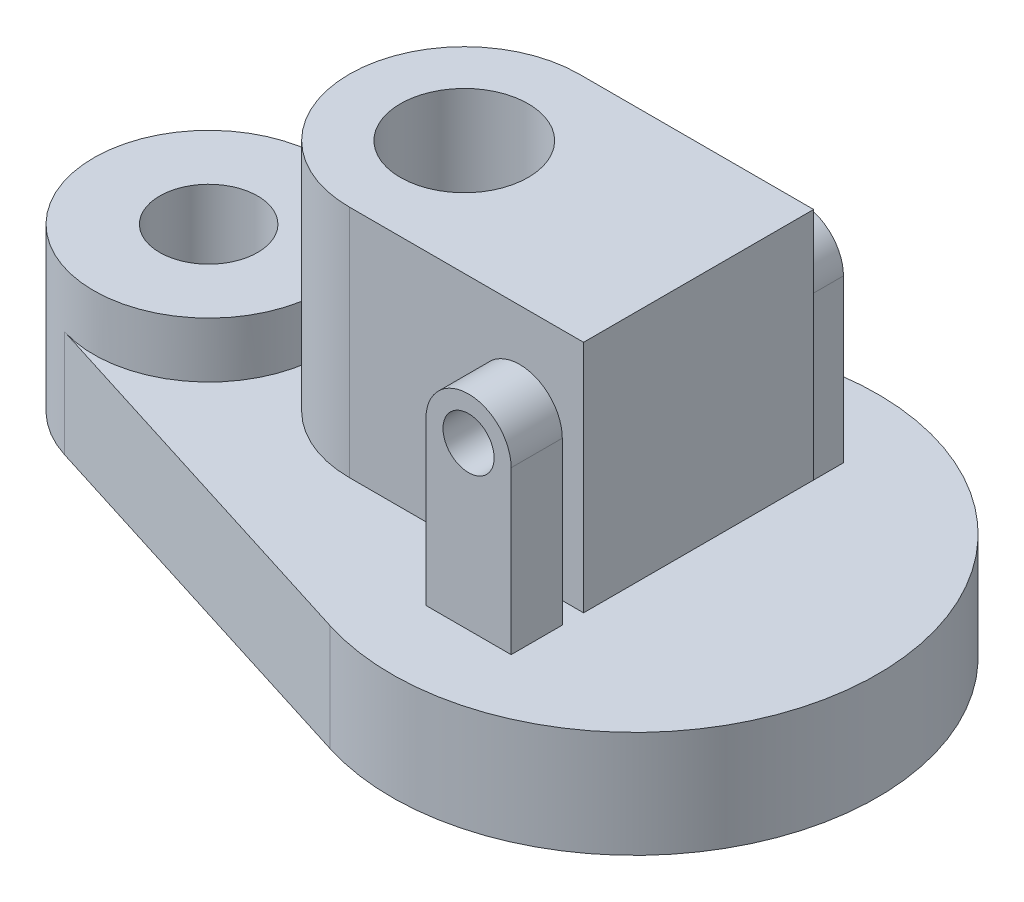
ISO-10303-21;
HEADER;
FILE_DESCRIPTION(('STEP AP214'),'2;1');
FILE_NAME('part.step','',(''),(''),'','','');
FILE_SCHEMA(('AUTOMOTIVE_DESIGN { 1 0 10303 214 1 1 1 1 }'));
ENDSEC;
DATA;
#1=APPLICATION_CONTEXT('core data for automotive mechanical design processes');
#2=APPLICATION_PROTOCOL_DEFINITION('international standard','automotive_design',2000,#1);
#3=PRODUCT_CONTEXT('',#1,'mechanical');
#4=PRODUCT('Part','Part','',(#3));
#5=PRODUCT_RELATED_PRODUCT_CATEGORY('part','',(#4));
#6=PRODUCT_DEFINITION_FORMATION('','',#4);
#7=PRODUCT_DEFINITION_CONTEXT('part definition',#1,'design');
#8=PRODUCT_DEFINITION('design','',#6,#7);
#9=PRODUCT_DEFINITION_SHAPE('','',#8);
#10=(LENGTH_UNIT() NAMED_UNIT(*) SI_UNIT(.MILLI.,.METRE.));
#11=(NAMED_UNIT(*) PLANE_ANGLE_UNIT() SI_UNIT($,.RADIAN.));
#12=(NAMED_UNIT(*) SI_UNIT($,.STERADIAN.) SOLID_ANGLE_UNIT());
#13=UNCERTAINTY_MEASURE_WITH_UNIT(LENGTH_MEASURE(1.E-05),#10,'distance_accuracy_value','');
#14=(GEOMETRIC_REPRESENTATION_CONTEXT(3) GLOBAL_UNCERTAINTY_ASSIGNED_CONTEXT((#13)) GLOBAL_UNIT_ASSIGNED_CONTEXT((#10,
#11,#12)) REPRESENTATION_CONTEXT('',''));
#15=CARTESIAN_POINT('',(0.,0.,0.));
#16=DIRECTION('',(0.,0.,1.));
#17=DIRECTION('',(1.,0.,0.));
#18=AXIS2_PLACEMENT_3D('',#15,#16,#17);
#19=CARTESIAN_POINT('',(0.,25.,0.));
#20=DIRECTION('',(0.,1.,0.));
#21=DIRECTION('',(0.,0.,1.));
#22=AXIS2_PLACEMENT_3D('',#19,#20,#21);
#23=PLANE('',#22);
#24=DIRECTION('',(0.953939201416946,0.,-0.3));
#25=VECTOR('',#24,1.);
#26=CARTESIAN_POINT('',(-17.1,25.,-54.3745344807659));
#27=LINE('',#26,#25);
#28=CARTESIAN_POINT('',(-108.1,25.,-25.7563584382575));
#29=VERTEX_POINT('',#28);
#30=CARTESIAN_POINT('',(-17.1,25.,-54.3745344807659));
#31=VERTEX_POINT('',#30);
#32=EDGE_CURVE('E247',#29,#31,#27,.T.);
#33=ORIENTED_EDGE('',*,*,#32,.F.);
#34=CARTESIAN_POINT('',(-100.,25.,0.));
#35=DIRECTION('',(0.,1.,0.));
#36=DIRECTION('',(0.,0.,1.));
#37=AXIS2_PLACEMENT_3D('',#34,#35,#36);
#38=CIRCLE('',#37,27.);
#39=CARTESIAN_POINT('',(-108.1,25.,25.7563584382575));
#40=VERTEX_POINT('',#39);
#41=EDGE_CURVE('E232',#29,#40,#38,.F.);
#42=ORIENTED_EDGE('',*,*,#41,.T.);
#43=DIRECTION('',(0.953939201416946,0.,0.3));
#44=VECTOR('',#43,1.);
#45=CARTESIAN_POINT('',(-17.1,25.,54.3745344807659));
#46=LINE('',#45,#44);
#47=CARTESIAN_POINT('',(-17.1,25.,54.3745344807659));
#48=VERTEX_POINT('',#47);
#49=EDGE_CURVE('E257',#40,#48,#46,.T.);
#50=ORIENTED_EDGE('',*,*,#49,.T.);
#51=CARTESIAN_POINT('',(0.,25.,0.));
#52=DIRECTION('',(0.,1.,0.));
#53=DIRECTION('',(0.,0.,1.));
#54=AXIS2_PLACEMENT_3D('',#51,#52,#53);
#55=CIRCLE('',#54,57.);
#56=EDGE_CURVE('E256',#48,#31,#55,.T.);
#57=ORIENTED_EDGE('',*,*,#56,.T.);
#58=EDGE_LOOP('',(#33,#42,#50,#57));
#59=FACE_BOUND('',#58,.T.);
#60=CARTESIAN_POINT('',(-40.,25.,0.));
#61=DIRECTION('',(0.,1.,0.));
#62=DIRECTION('',(0.,0.,1.));
#63=AXIS2_PLACEMENT_3D('',#60,#61,#62);
#64=CIRCLE('',#63,12.5);
#65=CARTESIAN_POINT('',(-40.,25.,12.5));
#66=VERTEX_POINT('',#65);
#67=EDGE_CURVE('E223',#66,#66,#64,.T.);
#68=ORIENTED_EDGE('',*,*,#67,.F.);
#69=EDGE_LOOP('',(#68));
#70=FACE_BOUND('',#69,.T.);
#71=DIRECTION('',(0.,0.,-1.));
#72=VECTOR('',#71,1.);
#73=CARTESIAN_POINT('',(10.,25.,39.));
#74=LINE('',#73,#72);
#75=CARTESIAN_POINT('',(10.,25.,39.));
#76=VERTEX_POINT('',#75);
#77=CARTESIAN_POINT('',(10.,25.,27.));
#78=VERTEX_POINT('',#77);
#79=EDGE_CURVE('E283',#76,#78,#74,.T.);
#80=ORIENTED_EDGE('',*,*,#79,.F.);
#81=DIRECTION('',(1.,0.,0.));
#82=VECTOR('',#81,1.);
#83=CARTESIAN_POINT('',(10.,25.,39.));
#84=LINE('',#83,#82);
#85=CARTESIAN_POINT('',(-10.,25.,39.));
#86=VERTEX_POINT('',#85);
#87=EDGE_CURVE('E282',#86,#76,#84,.T.);
#88=ORIENTED_EDGE('',*,*,#87,.F.);
#89=DIRECTION('',(0.,0.,-1.));
#90=VECTOR('',#89,1.);
#91=CARTESIAN_POINT('',(-10.,25.,39.));
#92=LINE('',#91,#90);
#93=CARTESIAN_POINT('',(-10.,25.,27.));
#94=VERTEX_POINT('',#93);
#95=EDGE_CURVE('E300',#86,#94,#92,.T.);
#96=ORIENTED_EDGE('',*,*,#95,.T.);
#97=DIRECTION('',(1.,0.,0.));
#98=VECTOR('',#97,1.);
#99=CARTESIAN_POINT('',(10.,25.,27.));
#100=LINE('',#99,#98);
#101=EDGE_CURVE('E280',#94,#78,#100,.T.);
#102=ORIENTED_EDGE('',*,*,#101,.T.);
#103=EDGE_LOOP('',(#80,#88,#96,#102));
#104=FACE_BOUND('',#103,.T.);
#105=DIRECTION('',(0.,0.,1.));
#106=VECTOR('',#105,1.);
#107=CARTESIAN_POINT('',(-9.99999999999999,25.,-39.));
#108=LINE('',#107,#106);
#109=CARTESIAN_POINT('',(-9.99999999999999,25.,-39.));
#110=VERTEX_POINT('',#109);
#111=CARTESIAN_POINT('',(-10.,25.,-27.));
#112=VERTEX_POINT('',#111);
#113=EDGE_CURVE('E218',#110,#112,#108,.T.);
#114=ORIENTED_EDGE('',*,*,#113,.F.);
#115=DIRECTION('',(1.,0.,0.));
#116=VECTOR('',#115,1.);
#117=CARTESIAN_POINT('',(-67.,25.,-39.));
#118=LINE('',#117,#116);
#119=CARTESIAN_POINT('',(9.99999999999999,25.,-39.));
#120=VERTEX_POINT('',#119);
#121=EDGE_CURVE('E187',#110,#120,#118,.T.);
#122=ORIENTED_EDGE('',*,*,#121,.T.);
#123=DIRECTION('',(0.,0.,1.));
#124=VECTOR('',#123,1.);
#125=CARTESIAN_POINT('',(9.99999999999999,25.,-39.));
#126=LINE('',#125,#124);
#127=CARTESIAN_POINT('',(9.99999999999999,25.,-27.));
#128=VERTEX_POINT('',#127);
#129=EDGE_CURVE('E199',#120,#128,#126,.T.);
#130=ORIENTED_EDGE('',*,*,#129,.T.);
#131=DIRECTION('',(1.,0.,0.));
#132=VECTOR('',#131,1.);
#133=CARTESIAN_POINT('',(-67.,25.,-27.));
#134=LINE('',#133,#132);
#135=EDGE_CURVE('E203',#112,#128,#134,.T.);
#136=ORIENTED_EDGE('',*,*,#135,.F.);
#137=EDGE_LOOP('',(#114,#122,#130,#136));
#138=FACE_BOUND('',#137,.T.);
#139=ADVANCED_FACE('F50',(#59,#70,#104,#138),#23,.T.);
#140=CARTESIAN_POINT('',(0.,85.,0.));
#141=DIRECTION('',(0.,-1.,0.));
#142=DIRECTION('',(0.,0.,-1.));
#143=AXIS2_PLACEMENT_3D('',#140,#141,#142);
#144=PLANE('',#143);
#145=CARTESIAN_POINT('',(-40.,85.,0.));
#146=DIRECTION('',(0.,1.,0.));
#147=DIRECTION('',(0.,0.,1.));
#148=AXIS2_PLACEMENT_3D('',#145,#146,#147);
#149=CIRCLE('',#148,15.);
#150=CARTESIAN_POINT('',(-40.,85.,15.));
#151=VERTEX_POINT('',#150);
#152=EDGE_CURVE('E308',#151,#151,#149,.T.);
#153=ORIENTED_EDGE('',*,*,#152,.F.);
#154=EDGE_LOOP('',(#153));
#155=FACE_BOUND('',#154,.T.);
#156=DIRECTION('',(-1.,0.,0.));
#157=VECTOR('',#156,1.);
#158=CARTESIAN_POINT('',(-67.,85.,-27.));
#159=LINE('',#158,#157);
#160=CARTESIAN_POINT('',(15.,85.,-27.));
#161=VERTEX_POINT('',#160);
#162=CARTESIAN_POINT('',(-40.,85.,-27.));
#163=VERTEX_POINT('',#162);
#164=EDGE_CURVE('E322',#161,#163,#159,.T.);
#165=ORIENTED_EDGE('',*,*,#164,.T.);
#166=CARTESIAN_POINT('',(-40.,85.,0.));
#167=DIRECTION('',(0.,-1.,0.));
#168=DIRECTION('',(0.,0.,-1.));
#169=AXIS2_PLACEMENT_3D('',#166,#167,#168);
#170=CIRCLE('',#169,27.);
#171=CARTESIAN_POINT('',(-67.,85.,0.));
#172=VERTEX_POINT('',#171);
#173=EDGE_CURVE('E342',#163,#172,#170,.F.);
#174=ORIENTED_EDGE('',*,*,#173,.T.);
#175=CARTESIAN_POINT('',(-40.,85.,0.));
#176=DIRECTION('',(0.,-1.,0.));
#177=DIRECTION('',(0.,0.,-1.));
#178=AXIS2_PLACEMENT_3D('',#175,#176,#177);
#179=CIRCLE('',#178,27.);
#180=CARTESIAN_POINT('',(-40.,85.,27.));
#181=VERTEX_POINT('',#180);
#182=EDGE_CURVE('E339',#172,#181,#179,.F.);
#183=ORIENTED_EDGE('',*,*,#182,.T.);
#184=DIRECTION('',(1.,0.,0.));
#185=VECTOR('',#184,1.);
#186=CARTESIAN_POINT('',(15.,85.,27.));
#187=LINE('',#186,#185);
#188=CARTESIAN_POINT('',(15.,85.,27.));
#189=VERTEX_POINT('',#188);
#190=EDGE_CURVE('E330',#181,#189,#187,.T.);
#191=ORIENTED_EDGE('',*,*,#190,.T.);
#192=DIRECTION('',(0.,0.,-1.));
#193=VECTOR('',#192,1.);
#194=CARTESIAN_POINT('',(15.,85.,-27.));
#195=LINE('',#194,#193);
#196=EDGE_CURVE('E328',#189,#161,#195,.T.);
#197=ORIENTED_EDGE('',*,*,#196,.T.);
#198=EDGE_LOOP('',(#165,#174,#183,#191,#197));
#199=FACE_BOUND('',#198,.T.);
#200=ADVANCED_FACE('F351',(#155,#199),#144,.F.);
#201=CARTESIAN_POINT('',(-40.,85.,0.));
#202=DIRECTION('',(0.,-1.,0.));
#203=DIRECTION('',(0.,0.,-1.));
#204=AXIS2_PLACEMENT_3D('',#201,#202,#203);
#205=CYLINDRICAL_SURFACE('',#204,27.);
#206=DIRECTION('',(0.,-1.,0.));
#207=VECTOR('',#206,1.);
#208=CARTESIAN_POINT('',(-40.,85.,-27.));
#209=LINE('',#208,#207);
#210=CARTESIAN_POINT('',(-40.,30.,-27.));
#211=VERTEX_POINT('',#210);
#212=EDGE_CURVE('E340',#211,#163,#209,.F.);
#213=ORIENTED_EDGE('',*,*,#212,.F.);
#214=CARTESIAN_POINT('',(-40.,30.,0.));
#215=DIRECTION('',(0.,-1.,0.));
#216=DIRECTION('',(0.,0.,-1.));
#217=AXIS2_PLACEMENT_3D('',#214,#215,#216);
#218=CIRCLE('',#217,27.);
#219=CARTESIAN_POINT('',(-67.,30.,0.));
#220=VERTEX_POINT('',#219);
#221=EDGE_CURVE('E11',#211,#220,#218,.F.);
#222=ORIENTED_EDGE('',*,*,#221,.T.);
#223=DIRECTION('',(0.,-1.,0.));
#224=VECTOR('',#223,1.);
#225=CARTESIAN_POINT('',(-67.,85.,0.));
#226=LINE('',#225,#224);
#227=EDGE_CURVE('E323',#220,#172,#226,.F.);
#228=ORIENTED_EDGE('',*,*,#227,.T.);
#229=ORIENTED_EDGE('',*,*,#173,.F.);
#230=EDGE_LOOP('',(#213,#222,#228,#229));
#231=FACE_BOUND('',#230,.T.);
#232=ADVANCED_FACE('F348',(#231),#205,.T.);
#233=CARTESIAN_POINT('',(-40.,85.,0.));
#234=DIRECTION('',(0.,-1.,0.));
#235=DIRECTION('',(0.,0.,-1.));
#236=AXIS2_PLACEMENT_3D('',#233,#234,#235);
#237=CYLINDRICAL_SURFACE('',#236,27.);
#238=ORIENTED_EDGE('',*,*,#227,.F.);
#239=CARTESIAN_POINT('',(-40.,30.,0.));
#240=DIRECTION('',(0.,-1.,0.));
#241=DIRECTION('',(0.,0.,-1.));
#242=AXIS2_PLACEMENT_3D('',#239,#240,#241);
#243=CIRCLE('',#242,27.);
#244=CARTESIAN_POINT('',(-40.,30.,27.));
#245=VERTEX_POINT('',#244);
#246=EDGE_CURVE('E319',#220,#245,#243,.F.);
#247=ORIENTED_EDGE('',*,*,#246,.T.);
#248=DIRECTION('',(0.,-1.,0.));
#249=VECTOR('',#248,1.);
#250=CARTESIAN_POINT('',(-40.,85.,27.));
#251=LINE('',#250,#249);
#252=EDGE_CURVE('E57',#181,#245,#251,.T.);
#253=ORIENTED_EDGE('',*,*,#252,.F.);
#254=ORIENTED_EDGE('',*,*,#182,.F.);
#255=EDGE_LOOP('',(#238,#247,#253,#254));
#256=FACE_BOUND('',#255,.T.);
#257=ADVANCED_FACE('F47',(#256),#237,.T.);
#258=CARTESIAN_POINT('',(15.,85.,-27.));
#259=DIRECTION('',(-1.,0.,0.));
#260=DIRECTION('',(0.,0.,1.));
#261=AXIS2_PLACEMENT_3D('',#258,#259,#260);
#262=PLANE('',#261);
#263=DIRECTION('',(0.,0.,-1.));
#264=VECTOR('',#263,1.);
#265=CARTESIAN_POINT('',(15.,30.,-27.));
#266=LINE('',#265,#264);
#267=CARTESIAN_POINT('',(15.,30.,27.));
#268=VERTEX_POINT('',#267);
#269=CARTESIAN_POINT('',(15.,30.,-27.));
#270=VERTEX_POINT('',#269);
#271=EDGE_CURVE('E316',#268,#270,#266,.T.);
#272=ORIENTED_EDGE('',*,*,#271,.T.);
#273=DIRECTION('',(0.,-1.,0.));
#274=VECTOR('',#273,1.);
#275=CARTESIAN_POINT('',(15.,85.,-27.));
#276=LINE('',#275,#274);
#277=EDGE_CURVE('E332',#161,#270,#276,.T.);
#278=ORIENTED_EDGE('',*,*,#277,.F.);
#279=ORIENTED_EDGE('',*,*,#196,.F.);
#280=DIRECTION('',(0.,-1.,0.));
#281=VECTOR('',#280,1.);
#282=CARTESIAN_POINT('',(15.,85.,27.));
#283=LINE('',#282,#281);
#284=EDGE_CURVE('E331',#189,#268,#283,.T.);
#285=ORIENTED_EDGE('',*,*,#284,.T.);
#286=EDGE_LOOP('',(#272,#278,#279,#285));
#287=FACE_BOUND('',#286,.T.);
#288=ADVANCED_FACE('F370',(#287),#262,.F.);
#289=CARTESIAN_POINT('',(15.,85.,27.));
#290=DIRECTION('',(0.,0.,-1.));
#291=DIRECTION('',(-1.,0.,0.));
#292=AXIS2_PLACEMENT_3D('',#289,#290,#291);
#293=PLANE('',#292);
#294=DIRECTION('',(0.,1.,0.));
#295=VECTOR('',#294,1.);
#296=CARTESIAN_POINT('',(10.,25.,27.));
#297=LINE('',#296,#295);
#298=CARTESIAN_POINT('',(10.,30.,27.));
#299=VERTEX_POINT('',#298);
#300=CARTESIAN_POINT('',(10.,63.,27.));
#301=VERTEX_POINT('',#300);
#302=EDGE_CURVE('E275',#299,#301,#297,.T.);
#303=ORIENTED_EDGE('',*,*,#302,.F.);
#304=DIRECTION('',(1.,0.,0.));
#305=VECTOR('',#304,1.);
#306=CARTESIAN_POINT('',(15.,30.,27.));
#307=LINE('',#306,#305);
#308=EDGE_CURVE('E313',#299,#268,#307,.T.);
#309=ORIENTED_EDGE('',*,*,#308,.T.);
#310=ORIENTED_EDGE('',*,*,#284,.F.);
#311=ORIENTED_EDGE('',*,*,#190,.F.);
#312=ORIENTED_EDGE('',*,*,#252,.T.);
#313=CARTESIAN_POINT('',(-10.,30.,27.));
#314=VERTEX_POINT('',#313);
#315=EDGE_CURVE('E311',#245,#314,#307,.T.);
#316=ORIENTED_EDGE('',*,*,#315,.T.);
#317=DIRECTION('',(0.,-1.,0.));
#318=VECTOR('',#317,1.);
#319=CARTESIAN_POINT('',(-10.,25.,27.));
#320=LINE('',#319,#318);
#321=CARTESIAN_POINT('',(-10.,63.,27.));
#322=VERTEX_POINT('',#321);
#323=EDGE_CURVE('E292',#322,#314,#320,.T.);
#324=ORIENTED_EDGE('',*,*,#323,.F.);
#325=CARTESIAN_POINT('',(0.,63.,27.));
#326=DIRECTION('',(0.,0.,1.));
#327=DIRECTION('',(-1.,0.,0.));
#328=AXIS2_PLACEMENT_3D('',#325,#326,#327);
#329=CIRCLE('',#328,10.);
#330=EDGE_CURVE('E290',#301,#322,#329,.T.);
#331=ORIENTED_EDGE('',*,*,#330,.F.);
#332=EDGE_LOOP('',(#303,#309,#310,#311,#312,#316,#324,#331));
#333=FACE_BOUND('',#332,.T.);
#334=ADVANCED_FACE('F363',(#333),#293,.F.);
#335=CARTESIAN_POINT('',(-67.,85.,-27.));
#336=DIRECTION('',(0.,0.,1.));
#337=DIRECTION('',(1.,0.,0.));
#338=AXIS2_PLACEMENT_3D('',#335,#336,#337);
#339=PLANE('',#338);
#340=DIRECTION('',(-1.,0.,0.));
#341=VECTOR('',#340,1.);
#342=CARTESIAN_POINT('',(-67.,30.,-27.));
#343=LINE('',#342,#341);
#344=CARTESIAN_POINT('',(10.,30.,-27.));
#345=VERTEX_POINT('',#344);
#346=EDGE_CURVE('E310',#270,#345,#343,.T.);
#347=ORIENTED_EDGE('',*,*,#346,.T.);
#348=DIRECTION('',(0.,1.,0.));
#349=VECTOR('',#348,1.);
#350=CARTESIAN_POINT('',(9.99999999999999,85.,-27.));
#351=LINE('',#350,#349);
#352=CARTESIAN_POINT('',(10.,63.,-27.));
#353=VERTEX_POINT('',#352);
#354=EDGE_CURVE('E68',#345,#353,#351,.T.);
#355=ORIENTED_EDGE('',*,*,#354,.T.);
#356=CARTESIAN_POINT('',(0.,63.,-27.));
#357=DIRECTION('',(0.,0.,1.));
#358=DIRECTION('',(1.,0.,0.));
#359=AXIS2_PLACEMENT_3D('',#356,#357,#358);
#360=CIRCLE('',#359,10.);
#361=CARTESIAN_POINT('',(-10.,63.,-27.));
#362=VERTEX_POINT('',#361);
#363=EDGE_CURVE('E63',#353,#362,#360,.T.);
#364=ORIENTED_EDGE('',*,*,#363,.T.);
#365=DIRECTION('',(0.,-1.,0.));
#366=VECTOR('',#365,1.);
#367=CARTESIAN_POINT('',(-10.,85.,-27.));
#368=LINE('',#367,#366);
#369=CARTESIAN_POINT('',(-9.99999999999999,30.,-27.));
#370=VERTEX_POINT('',#369);
#371=EDGE_CURVE('E204',#362,#370,#368,.T.);
#372=ORIENTED_EDGE('',*,*,#371,.T.);
#373=EDGE_CURVE('E315',#370,#211,#343,.T.);
#374=ORIENTED_EDGE('',*,*,#373,.T.);
#375=ORIENTED_EDGE('',*,*,#212,.T.);
#376=ORIENTED_EDGE('',*,*,#164,.F.);
#377=ORIENTED_EDGE('',*,*,#277,.T.);
#378=EDGE_LOOP('',(#347,#355,#364,#372,#374,#375,#376,#377));
#379=FACE_BOUND('',#378,.T.);
#380=ADVANCED_FACE('F369',(#379),#339,.F.);
#381=CARTESIAN_POINT('',(0.,30.,0.));
#382=DIRECTION('',(0.,-1.,0.));
#383=DIRECTION('',(0.,0.,-1.));
#384=AXIS2_PLACEMENT_3D('',#381,#382,#383);
#385=PLANE('',#384);
#386=CARTESIAN_POINT('',(-40.,30.,0.));
#387=DIRECTION('',(0.,-1.,0.));
#388=DIRECTION('',(0.,0.,-1.));
#389=AXIS2_PLACEMENT_3D('',#386,#387,#388);
#390=CIRCLE('',#389,15.);
#391=CARTESIAN_POINT('',(-40.,30.,-15.));
#392=VERTEX_POINT('',#391);
#393=EDGE_CURVE('E51',#392,#392,#390,.T.);
#394=ORIENTED_EDGE('',*,*,#393,.F.);
#395=EDGE_LOOP('',(#394));
#396=FACE_BOUND('',#395,.T.);
#397=ORIENTED_EDGE('',*,*,#221,.F.);
#398=ORIENTED_EDGE('',*,*,#373,.F.);
#399=DIRECTION('',(-1.,0.,0.));
#400=VECTOR('',#399,1.);
#401=CARTESIAN_POINT('',(0.,30.,-27.));
#402=LINE('',#401,#400);
#403=EDGE_CURVE('E217',#345,#370,#402,.T.);
#404=ORIENTED_EDGE('',*,*,#403,.F.);
#405=ORIENTED_EDGE('',*,*,#346,.F.);
#406=ORIENTED_EDGE('',*,*,#271,.F.);
#407=ORIENTED_EDGE('',*,*,#308,.F.);
#408=EDGE_CURVE('E320',#314,#299,#307,.T.);
#409=ORIENTED_EDGE('',*,*,#408,.F.);
#410=ORIENTED_EDGE('',*,*,#315,.F.);
#411=ORIENTED_EDGE('',*,*,#246,.F.);
#412=EDGE_LOOP('',(#397,#398,#404,#405,#406,#407,#409,#410,#411));
#413=FACE_BOUND('',#412,.T.);
#414=ADVANCED_FACE('F375',(#396,#413),#385,.T.);
#415=CARTESIAN_POINT('',(-40.,-17.4264068711928,0.));
#416=DIRECTION('',(0.,1.,0.));
#417=DIRECTION('',(0.,0.,1.));
#418=AXIS2_PLACEMENT_3D('',#415,#416,#417);
#419=CYLINDRICAL_SURFACE('',#418,15.);
#420=ORIENTED_EDGE('',*,*,#393,.T.);
#421=EDGE_LOOP('',(#420));
#422=FACE_BOUND('',#421,.T.);
#423=ORIENTED_EDGE('',*,*,#152,.T.);
#424=EDGE_LOOP('',(#423));
#425=FACE_BOUND('',#424,.T.);
#426=ADVANCED_FACE('F424',(#422,#425),#419,.F.);
#427=CARTESIAN_POINT('',(0.,63.,39.));
#428=DIRECTION('',(0.,0.,-1.));
#429=DIRECTION('',(-1.,0.,0.));
#430=AXIS2_PLACEMENT_3D('',#427,#428,#429);
#431=PLANE('',#430);
#432=DIRECTION('',(0.,1.,0.));
#433=VECTOR('',#432,1.);
#434=CARTESIAN_POINT('',(10.,25.,39.));
#435=LINE('',#434,#433);
#436=CARTESIAN_POINT('',(10.,63.,39.));
#437=VERTEX_POINT('',#436);
#438=EDGE_CURVE('E272',#76,#437,#435,.T.);
#439=ORIENTED_EDGE('',*,*,#438,.T.);
#440=CARTESIAN_POINT('',(0.,63.,39.));
#441=DIRECTION('',(0.,0.,1.));
#442=DIRECTION('',(-1.,0.,0.));
#443=AXIS2_PLACEMENT_3D('',#440,#441,#442);
#444=CIRCLE('',#443,10.);
#445=CARTESIAN_POINT('',(-10.,63.,39.));
#446=VERTEX_POINT('',#445);
#447=EDGE_CURVE('E277',#437,#446,#444,.T.);
#448=ORIENTED_EDGE('',*,*,#447,.T.);
#449=DIRECTION('',(0.,-1.,0.));
#450=VECTOR('',#449,1.);
#451=CARTESIAN_POINT('',(-10.,25.,39.));
#452=LINE('',#451,#450);
#453=EDGE_CURVE('E276',#446,#86,#452,.T.);
#454=ORIENTED_EDGE('',*,*,#453,.T.);
#455=ORIENTED_EDGE('',*,*,#87,.T.);
#456=EDGE_LOOP('',(#439,#448,#454,#455));
#457=FACE_BOUND('',#456,.T.);
#458=CARTESIAN_POINT('',(0.,63.,39.));
#459=DIRECTION('',(0.,0.,1.));
#460=DIRECTION('',(1.,0.,0.));
#461=AXIS2_PLACEMENT_3D('',#458,#459,#460);
#462=CIRCLE('',#461,6.);
#463=CARTESIAN_POINT('',(6.,63.,39.));
#464=VERTEX_POINT('',#463);
#465=EDGE_CURVE('E270',#464,#464,#462,.T.);
#466=ORIENTED_EDGE('',*,*,#465,.F.);
#467=EDGE_LOOP('',(#466));
#468=FACE_BOUND('',#467,.T.);
#469=ADVANCED_FACE('F419',(#457,#468),#431,.F.);
#470=CARTESIAN_POINT('',(0.,63.,27.));
#471=DIRECTION('',(0.,0.,-1.));
#472=DIRECTION('',(-1.,0.,0.));
#473=AXIS2_PLACEMENT_3D('',#470,#471,#472);
#474=PLANE('',#473);
#475=EDGE_CURVE('E286',#314,#94,#320,.T.);
#476=ORIENTED_EDGE('',*,*,#475,.F.);
#477=ORIENTED_EDGE('',*,*,#408,.T.);
#478=EDGE_CURVE('E284',#78,#299,#297,.T.);
#479=ORIENTED_EDGE('',*,*,#478,.F.);
#480=ORIENTED_EDGE('',*,*,#101,.F.);
#481=EDGE_LOOP('',(#476,#477,#479,#480));
#482=FACE_BOUND('',#481,.T.);
#483=ADVANCED_FACE('F421',(#482),#474,.T.);
#484=CARTESIAN_POINT('',(10.,25.,39.));
#485=DIRECTION('',(-1.,0.,0.));
#486=DIRECTION('',(0.,-1.,0.));
#487=AXIS2_PLACEMENT_3D('',#484,#485,#486);
#488=PLANE('',#487);
#489=ORIENTED_EDGE('',*,*,#478,.T.);
#490=ORIENTED_EDGE('',*,*,#302,.T.);
#491=DIRECTION('',(0.,0.,-1.));
#492=VECTOR('',#491,1.);
#493=CARTESIAN_POINT('',(10.,63.,39.));
#494=LINE('',#493,#492);
#495=EDGE_CURVE('E303',#437,#301,#494,.T.);
#496=ORIENTED_EDGE('',*,*,#495,.F.);
#497=ORIENTED_EDGE('',*,*,#438,.F.);
#498=ORIENTED_EDGE('',*,*,#79,.T.);
#499=EDGE_LOOP('',(#489,#490,#496,#497,#498));
#500=FACE_BOUND('',#499,.T.);
#501=ADVANCED_FACE('F428',(#500),#488,.F.);
#502=CARTESIAN_POINT('',(0.,63.,39.));
#503=DIRECTION('',(0.,0.,-1.));
#504=DIRECTION('',(-1.,0.,0.));
#505=AXIS2_PLACEMENT_3D('',#502,#503,#504);
#506=CYLINDRICAL_SURFACE('',#505,10.);
#507=ORIENTED_EDGE('',*,*,#330,.T.);
#508=DIRECTION('',(0.,0.,-1.));
#509=VECTOR('',#508,1.);
#510=CARTESIAN_POINT('',(-10.,63.,39.));
#511=LINE('',#510,#509);
#512=EDGE_CURVE('E296',#446,#322,#511,.T.);
#513=ORIENTED_EDGE('',*,*,#512,.F.);
#514=ORIENTED_EDGE('',*,*,#447,.F.);
#515=ORIENTED_EDGE('',*,*,#495,.T.);
#516=EDGE_LOOP('',(#507,#513,#514,#515));
#517=FACE_BOUND('',#516,.T.);
#518=ADVANCED_FACE('F431',(#517),#506,.T.);
#519=CARTESIAN_POINT('',(-10.,25.,39.));
#520=DIRECTION('',(1.,0.,0.));
#521=DIRECTION('',(0.,1.,0.));
#522=AXIS2_PLACEMENT_3D('',#519,#520,#521);
#523=PLANE('',#522);
#524=ORIENTED_EDGE('',*,*,#323,.T.);
#525=ORIENTED_EDGE('',*,*,#475,.T.);
#526=ORIENTED_EDGE('',*,*,#95,.F.);
#527=ORIENTED_EDGE('',*,*,#453,.F.);
#528=ORIENTED_EDGE('',*,*,#512,.T.);
#529=EDGE_LOOP('',(#524,#525,#526,#527,#528));
#530=FACE_BOUND('',#529,.T.);
#531=ADVANCED_FACE('F416',(#530),#523,.F.);
#532=CARTESIAN_POINT('',(0.,63.,39.));
#533=DIRECTION('',(0.,0.,-1.));
#534=DIRECTION('',(-1.,0.,0.));
#535=AXIS2_PLACEMENT_3D('',#532,#533,#534);
#536=CYLINDRICAL_SURFACE('',#535,6.);
#537=ORIENTED_EDGE('',*,*,#465,.T.);
#538=EDGE_LOOP('',(#537));
#539=FACE_BOUND('',#538,.T.);
#540=CARTESIAN_POINT('',(0.,63.,-39.));
#541=DIRECTION('',(0.,0.,1.));
#542=DIRECTION('',(1.,0.,0.));
#543=AXIS2_PLACEMENT_3D('',#540,#541,#542);
#544=CIRCLE('',#543,6.);
#545=CARTESIAN_POINT('',(6.,63.,-39.));
#546=VERTEX_POINT('',#545);
#547=EDGE_CURVE('E210',#546,#546,#544,.T.);
#548=ORIENTED_EDGE('',*,*,#547,.F.);
#549=EDGE_LOOP('',(#548));
#550=FACE_BOUND('',#549,.T.);
#551=ADVANCED_FACE('F414',(#539,#550),#536,.F.);
#552=CARTESIAN_POINT('',(-17.1,25.,-54.3745344807659));
#553=DIRECTION('',(-0.3,0.,-0.953939201416946));
#554=DIRECTION('',(-0.953939201416946,0.,0.3));
#555=AXIS2_PLACEMENT_3D('',#552,#553,#554);
#556=PLANE('',#555);
#557=DIRECTION('',(0.953939201416946,0.,-0.3));
#558=VECTOR('',#557,1.);
#559=CARTESIAN_POINT('',(-17.1,0.,-54.3745344807659));
#560=LINE('',#559,#558);
#561=CARTESIAN_POINT('',(-108.1,0.,-25.7563584382575));
#562=VERTEX_POINT('',#561);
#563=CARTESIAN_POINT('',(-17.1,0.,-54.3745344807659));
#564=VERTEX_POINT('',#563);
#565=EDGE_CURVE('E253',#562,#564,#560,.T.);
#566=ORIENTED_EDGE('',*,*,#565,.F.);
#567=DIRECTION('',(0.,-1.,0.));
#568=VECTOR('',#567,1.);
#569=CARTESIAN_POINT('',(-108.1,25.,-25.7563584382575));
#570=LINE('',#569,#568);
#571=EDGE_CURVE('E235',#29,#562,#570,.T.);
#572=ORIENTED_EDGE('',*,*,#571,.F.);
#573=ORIENTED_EDGE('',*,*,#32,.T.);
#574=DIRECTION('',(0.,-1.,0.));
#575=VECTOR('',#574,1.);
#576=CARTESIAN_POINT('',(-17.1,25.,-54.3745344807659));
#577=LINE('',#576,#575);
#578=EDGE_CURVE('E244',#31,#564,#577,.T.);
#579=ORIENTED_EDGE('',*,*,#578,.T.);
#580=EDGE_LOOP('',(#566,#572,#573,#579));
#581=FACE_BOUND('',#580,.T.);
#582=ADVANCED_FACE('F417',(#581),#556,.T.);
#583=CARTESIAN_POINT('',(-100.,25.,0.));
#584=DIRECTION('',(0.,-1.,0.));
#585=DIRECTION('',(0.,0.,-1.));
#586=AXIS2_PLACEMENT_3D('',#583,#584,#585);
#587=CYLINDRICAL_SURFACE('',#586,27.);
#588=CARTESIAN_POINT('',(-100.,0.,0.));
#589=DIRECTION('',(0.,1.,0.));
#590=DIRECTION('',(0.,0.,1.));
#591=AXIS2_PLACEMENT_3D('',#588,#589,#590);
#592=CIRCLE('',#591,27.);
#593=CARTESIAN_POINT('',(-108.1,0.,25.7563584382575));
#594=VERTEX_POINT('',#593);
#595=EDGE_CURVE('E231',#562,#594,#592,.T.);
#596=ORIENTED_EDGE('',*,*,#595,.T.);
#597=DIRECTION('',(0.,-1.,0.));
#598=VECTOR('',#597,1.);
#599=CARTESIAN_POINT('',(-108.1,25.,25.7563584382575));
#600=LINE('',#599,#598);
#601=EDGE_CURVE('E237',#40,#594,#600,.T.);
#602=ORIENTED_EDGE('',*,*,#601,.F.);
#603=ORIENTED_EDGE('',*,*,#41,.F.);
#604=ORIENTED_EDGE('',*,*,#571,.T.);
#605=EDGE_LOOP('',(#596,#602,#603,#604));
#606=FACE_BOUND('',#605,.T.);
#607=CARTESIAN_POINT('',(-100.,38.,0.));
#608=DIRECTION('',(0.,1.,0.));
#609=DIRECTION('',(0.,0.,1.));
#610=AXIS2_PLACEMENT_3D('',#607,#608,#609);
#611=CIRCLE('',#610,27.);
#612=CARTESIAN_POINT('',(-100.,38.,27.));
#613=VERTEX_POINT('',#612);
#614=EDGE_CURVE('E246',#613,#613,#611,.T.);
#615=ORIENTED_EDGE('',*,*,#614,.F.);
#616=EDGE_LOOP('',(#615));
#617=FACE_BOUND('',#616,.T.);
#618=ADVANCED_FACE('F482',(#606,#617),#587,.T.);
#619=CARTESIAN_POINT('',(-17.1,25.,54.3745344807659));
#620=DIRECTION('',(0.3,0.,-0.953939201416946));
#621=DIRECTION('',(-0.953939201416946,0.,-0.3));
#622=AXIS2_PLACEMENT_3D('',#619,#620,#621);
#623=PLANE('',#622);
#624=DIRECTION('',(0.953939201416946,0.,0.3));
#625=VECTOR('',#624,1.);
#626=CARTESIAN_POINT('',(-17.1,0.,54.3745344807659));
#627=LINE('',#626,#625);
#628=CARTESIAN_POINT('',(-17.1,0.,54.3745344807659));
#629=VERTEX_POINT('',#628);
#630=EDGE_CURVE('E234',#594,#629,#627,.T.);
#631=ORIENTED_EDGE('',*,*,#630,.T.);
#632=DIRECTION('',(0.,-1.,0.));
#633=VECTOR('',#632,1.);
#634=CARTESIAN_POINT('',(-17.1,25.,54.3745344807659));
#635=LINE('',#634,#633);
#636=EDGE_CURVE('E238',#48,#629,#635,.T.);
#637=ORIENTED_EDGE('',*,*,#636,.F.);
#638=ORIENTED_EDGE('',*,*,#49,.F.);
#639=ORIENTED_EDGE('',*,*,#601,.T.);
#640=EDGE_LOOP('',(#631,#637,#638,#639));
#641=FACE_BOUND('',#640,.T.);
#642=ADVANCED_FACE('F490',(#641),#623,.F.);
#643=CARTESIAN_POINT('',(0.,25.,0.));
#644=DIRECTION('',(0.,-1.,0.));
#645=DIRECTION('',(0.,0.,-1.));
#646=AXIS2_PLACEMENT_3D('',#643,#644,#645);
#647=CYLINDRICAL_SURFACE('',#646,57.);
#648=CARTESIAN_POINT('',(0.,0.,0.));
#649=DIRECTION('',(0.,1.,0.));
#650=DIRECTION('',(0.,0.,1.));
#651=AXIS2_PLACEMENT_3D('',#648,#649,#650);
#652=CIRCLE('',#651,57.);
#653=EDGE_CURVE('E239',#629,#564,#652,.T.);
#654=ORIENTED_EDGE('',*,*,#653,.T.);
#655=ORIENTED_EDGE('',*,*,#578,.F.);
#656=ORIENTED_EDGE('',*,*,#56,.F.);
#657=ORIENTED_EDGE('',*,*,#636,.T.);
#658=EDGE_LOOP('',(#654,#655,#656,#657));
#659=FACE_BOUND('',#658,.T.);
#660=ADVANCED_FACE('F494',(#659),#647,.T.);
#661=CARTESIAN_POINT('',(-100.,25.,0.));
#662=DIRECTION('',(0.,-1.,0.));
#663=DIRECTION('',(0.,0.,-1.));
#664=AXIS2_PLACEMENT_3D('',#661,#662,#663);
#665=CYLINDRICAL_SURFACE('',#664,11.5);
#666=CARTESIAN_POINT('',(-100.,0.,0.));
#667=DIRECTION('',(0.,1.,0.));
#668=DIRECTION('',(0.,0.,1.));
#669=AXIS2_PLACEMENT_3D('',#666,#667,#668);
#670=CIRCLE('',#669,11.5);
#671=CARTESIAN_POINT('',(-100.,0.,11.5));
#672=VERTEX_POINT('',#671);
#673=EDGE_CURVE('E250',#672,#672,#670,.T.);
#674=ORIENTED_EDGE('',*,*,#673,.F.);
#675=EDGE_LOOP('',(#674));
#676=FACE_BOUND('',#675,.T.);
#677=CARTESIAN_POINT('',(-100.,38.,0.));
#678=DIRECTION('',(0.,1.,0.));
#679=DIRECTION('',(0.,0.,1.));
#680=AXIS2_PLACEMENT_3D('',#677,#678,#679);
#681=CIRCLE('',#680,11.5);
#682=CARTESIAN_POINT('',(-100.,38.,11.5));
#683=VERTEX_POINT('',#682);
#684=EDGE_CURVE('E243',#683,#683,#681,.T.);
#685=ORIENTED_EDGE('',*,*,#684,.T.);
#686=EDGE_LOOP('',(#685));
#687=FACE_BOUND('',#686,.T.);
#688=ADVANCED_FACE('F492',(#676,#687),#665,.F.);
#689=CARTESIAN_POINT('',(0.,0.,0.));
#690=DIRECTION('',(0.,1.,0.));
#691=DIRECTION('',(0.,0.,1.));
#692=AXIS2_PLACEMENT_3D('',#689,#690,#691);
#693=PLANE('',#692);
#694=CARTESIAN_POINT('',(-40.,0.,0.));
#695=DIRECTION('',(0.,1.,0.));
#696=DIRECTION('',(0.,0.,1.));
#697=AXIS2_PLACEMENT_3D('',#694,#695,#696);
#698=CIRCLE('',#697,12.5);
#699=CARTESIAN_POINT('',(-40.,0.,12.5));
#700=VERTEX_POINT('',#699);
#701=EDGE_CURVE('E228',#700,#700,#698,.F.);
#702=ORIENTED_EDGE('',*,*,#701,.F.);
#703=EDGE_LOOP('',(#702));
#704=FACE_BOUND('',#703,.T.);
#705=ORIENTED_EDGE('',*,*,#630,.F.);
#706=ORIENTED_EDGE('',*,*,#595,.F.);
#707=ORIENTED_EDGE('',*,*,#565,.T.);
#708=ORIENTED_EDGE('',*,*,#653,.F.);
#709=EDGE_LOOP('',(#705,#706,#707,#708));
#710=FACE_BOUND('',#709,.T.);
#711=ORIENTED_EDGE('',*,*,#673,.T.);
#712=EDGE_LOOP('',(#711));
#713=FACE_BOUND('',#712,.T.);
#714=ADVANCED_FACE('F408',(#704,#710,#713),#693,.F.);
#715=CARTESIAN_POINT('',(0.,38.,0.));
#716=DIRECTION('',(0.,1.,0.));
#717=DIRECTION('',(0.,0.,1.));
#718=AXIS2_PLACEMENT_3D('',#715,#716,#717);
#719=PLANE('',#718);
#720=ORIENTED_EDGE('',*,*,#684,.F.);
#721=EDGE_LOOP('',(#720));
#722=FACE_BOUND('',#721,.T.);
#723=ORIENTED_EDGE('',*,*,#614,.T.);
#724=EDGE_LOOP('',(#723));
#725=FACE_BOUND('',#724,.T.);
#726=ADVANCED_FACE('F406',(#722,#725),#719,.T.);
#727=CARTESIAN_POINT('',(-40.,-35.3553390593274,0.));
#728=DIRECTION('',(0.,1.,0.));
#729=DIRECTION('',(0.,0.,1.));
#730=AXIS2_PLACEMENT_3D('',#727,#728,#729);
#731=CYLINDRICAL_SURFACE('',#730,12.5);
#732=CARTESIAN_POINT('',(-40.,0.,12.5));
#733=CARTESIAN_POINT('',(-40.,0.260416666666659,12.5));
#734=CARTESIAN_POINT('',(-40.,0.520833333333325,12.5));
#735=CARTESIAN_POINT('',(-40.,1.04166666666666,12.5));
#736=CARTESIAN_POINT('',(-40.,1.30208333333333,12.5));
#737=CARTESIAN_POINT('',(-40.,1.82291666666666,12.5));
#738=CARTESIAN_POINT('',(-40.,2.08333333333333,12.5));
#739=CARTESIAN_POINT('',(-40.,2.60416666666666,12.5));
#740=CARTESIAN_POINT('',(-40.,2.86458333333333,12.5));
#741=CARTESIAN_POINT('',(-40.,3.38541666666666,12.5));
#742=CARTESIAN_POINT('',(-40.,3.64583333333333,12.5));
#743=CARTESIAN_POINT('',(-40.,4.16666666666666,12.5));
#744=CARTESIAN_POINT('',(-40.,4.42708333333333,12.5));
#745=CARTESIAN_POINT('',(-40.,4.94791666666666,12.5));
#746=CARTESIAN_POINT('',(-40.,5.20833333333333,12.5));
#747=CARTESIAN_POINT('',(-40.,5.72916666666666,12.5));
#748=CARTESIAN_POINT('',(-40.,5.98958333333333,12.5));
#749=CARTESIAN_POINT('',(-40.,6.51041666666666,12.5));
#750=CARTESIAN_POINT('',(-40.,6.77083333333333,12.5));
#751=CARTESIAN_POINT('',(-40.,7.29166666666666,12.5));
#752=CARTESIAN_POINT('',(-40.,7.55208333333333,12.5));
#753=CARTESIAN_POINT('',(-40.,8.07291666666666,12.5));
#754=CARTESIAN_POINT('',(-40.,8.33333333333333,12.5));
#755=CARTESIAN_POINT('',(-40.,8.85416666666666,12.5));
#756=CARTESIAN_POINT('',(-40.,9.11458333333333,12.5));
#757=CARTESIAN_POINT('',(-40.,9.63541666666666,12.5));
#758=CARTESIAN_POINT('',(-40.,9.89583333333333,12.5));
#759=CARTESIAN_POINT('',(-40.,10.4166666666667,12.5));
#760=CARTESIAN_POINT('',(-40.,10.6770833333333,12.5));
#761=CARTESIAN_POINT('',(-40.,11.1979166666667,12.5));
#762=CARTESIAN_POINT('',(-40.,11.4583333333333,12.5));
#763=CARTESIAN_POINT('',(-40.,11.9791666666667,12.5));
#764=CARTESIAN_POINT('',(-40.,12.2395833333333,12.5));
#765=CARTESIAN_POINT('',(-40.,12.7604166666667,12.5));
#766=CARTESIAN_POINT('',(-40.,13.0208333333333,12.5));
#767=CARTESIAN_POINT('',(-40.,13.5416666666667,12.5));
#768=CARTESIAN_POINT('',(-40.,13.8020833333333,12.5));
#769=CARTESIAN_POINT('',(-40.,14.3229166666667,12.5));
#770=CARTESIAN_POINT('',(-40.,14.5833333333333,12.5));
#771=CARTESIAN_POINT('',(-40.,15.1041666666667,12.5));
#772=CARTESIAN_POINT('',(-40.,15.3645833333333,12.5));
#773=CARTESIAN_POINT('',(-40.,15.8854166666667,12.5));
#774=CARTESIAN_POINT('',(-40.,16.1458333333333,12.5));
#775=CARTESIAN_POINT('',(-40.,16.6666666666667,12.5));
#776=CARTESIAN_POINT('',(-40.,16.9270833333333,12.5));
#777=CARTESIAN_POINT('',(-40.,17.4479166666667,12.5));
#778=CARTESIAN_POINT('',(-40.,17.7083333333333,12.5));
#779=CARTESIAN_POINT('',(-40.,18.2291666666667,12.5));
#780=CARTESIAN_POINT('',(-40.,18.4895833333333,12.5));
#781=CARTESIAN_POINT('',(-40.,19.0104166666667,12.5));
#782=CARTESIAN_POINT('',(-40.,19.2708333333333,12.5));
#783=CARTESIAN_POINT('',(-40.,19.7916666666667,12.5));
#784=CARTESIAN_POINT('',(-40.,20.0520833333333,12.5));
#785=CARTESIAN_POINT('',(-40.,20.5729166666667,12.5));
#786=CARTESIAN_POINT('',(-40.,20.8333333333333,12.5));
#787=CARTESIAN_POINT('',(-40.,21.3541666666667,12.5));
#788=CARTESIAN_POINT('',(-40.,21.6145833333333,12.5));
#789=CARTESIAN_POINT('',(-40.,22.1354166666667,12.5));
#790=CARTESIAN_POINT('',(-40.,22.3958333333333,12.5));
#791=CARTESIAN_POINT('',(-40.,22.9166666666667,12.5));
#792=CARTESIAN_POINT('',(-40.,23.1770833333333,12.5));
#793=CARTESIAN_POINT('',(-40.,23.6979166666667,12.5));
#794=CARTESIAN_POINT('',(-40.,23.9583333333333,12.5));
#795=CARTESIAN_POINT('',(-40.,24.4791666666667,12.5));
#796=CARTESIAN_POINT('',(-40.,24.7395833333333,12.5));
#797=CARTESIAN_POINT('',(-40.,25.,12.5));
#798=B_SPLINE_CURVE_WITH_KNOTS('',3,(#732,#733,#734,#735,#736,#737,#738,#739,#740,#741,#742,
#743,#744,#745,#746,#747,#748,#749,#750,#751,#752,#753,#754,#755,#756,#757,#758,#759,#760,#761,
#762,#763,#764,#765,#766,#767,#768,#769,#770,#771,#772,#773,#774,#775,#776,#777,#778,#779,#780,
#781,#782,#783,#784,#785,#786,#787,#788,#789,#790,#791,#792,#793,#794,#795,#796,#797),
.UNSPECIFIED.,.F.,.F.,(4,2,2,2,2,2,2,2,2,2,2,2,2,2,2,2,2,2,2,2,2,2,2,2,2,2,2,2,2,2,2,2,4),(0.,
0.781249999999997,1.5625,2.34375,3.125,3.90625,4.6875,5.46875,6.25000000000001,7.03125,7.8125,
8.59375,9.375,10.15625,10.9375,11.71875,12.5,13.28125,14.0625,14.84375,15.625,16.40625,17.1875,
17.96875,18.75,19.53125,20.3125,21.09375,21.875,22.65625,23.4375,24.21875,25.),.UNSPECIFIED.);
#799=EDGE_CURVE('BSEAM392',#700,#66,#798,.T.);
#800=ORIENTED_EDGE('',*,*,#701,.T.);
#801=ORIENTED_EDGE('',*,*,#67,.T.);
#802=ORIENTED_EDGE('',*,*,#799,.T.);
#803=ORIENTED_EDGE('',*,*,#799,.F.);
#804=EDGE_LOOP('',(#800,#802,#801,#803));
#805=FACE_BOUND('',#804,.T.);
#806=ADVANCED_FACE('F392',(#805),#731,.F.);
#807=CARTESIAN_POINT('',(9.99999999999999,85.,-39.));
#808=DIRECTION('',(1.,0.,0.));
#809=DIRECTION('',(0.,1.,0.));
#810=AXIS2_PLACEMENT_3D('',#807,#808,#809);
#811=PLANE('',#810);
#812=EDGE_CURVE('E211',#128,#345,#351,.T.);
#813=ORIENTED_EDGE('',*,*,#812,.F.);
#814=ORIENTED_EDGE('',*,*,#129,.F.);
#815=DIRECTION('',(0.,1.,0.));
#816=VECTOR('',#815,1.);
#817=CARTESIAN_POINT('',(9.99999999999999,85.,-39.));
#818=LINE('',#817,#816);
#819=CARTESIAN_POINT('',(10.,63.,-39.));
#820=VERTEX_POINT('',#819);
#821=EDGE_CURVE('E193',#120,#820,#818,.T.);
#822=ORIENTED_EDGE('',*,*,#821,.T.);
#823=DIRECTION('',(0.,0.,1.));
#824=VECTOR('',#823,1.);
#825=CARTESIAN_POINT('',(10.,63.,-39.));
#826=LINE('',#825,#824);
#827=EDGE_CURVE('E179',#820,#353,#826,.T.);
#828=ORIENTED_EDGE('',*,*,#827,.T.);
#829=ORIENTED_EDGE('',*,*,#354,.F.);
#830=EDGE_LOOP('',(#813,#814,#822,#828,#829));
#831=FACE_BOUND('',#830,.T.);
#832=ADVANCED_FACE('F200',(#831),#811,.T.);
#833=CARTESIAN_POINT('',(-10.,85.,-39.));
#834=DIRECTION('',(-1.,0.,0.));
#835=DIRECTION('',(0.,-1.,0.));
#836=AXIS2_PLACEMENT_3D('',#833,#834,#835);
#837=PLANE('',#836);
#838=ORIENTED_EDGE('',*,*,#371,.F.);
#839=DIRECTION('',(0.,0.,1.));
#840=VECTOR('',#839,1.);
#841=CARTESIAN_POINT('',(-10.,63.,-39.));
#842=LINE('',#841,#840);
#843=CARTESIAN_POINT('',(-10.,63.,-39.));
#844=VERTEX_POINT('',#843);
#845=EDGE_CURVE('E183',#844,#362,#842,.T.);
#846=ORIENTED_EDGE('',*,*,#845,.F.);
#847=DIRECTION('',(0.,-1.,0.));
#848=VECTOR('',#847,1.);
#849=CARTESIAN_POINT('',(-10.,85.,-39.));
#850=LINE('',#849,#848);
#851=EDGE_CURVE('E191',#844,#110,#850,.T.);
#852=ORIENTED_EDGE('',*,*,#851,.T.);
#853=ORIENTED_EDGE('',*,*,#113,.T.);
#854=EDGE_CURVE('E214',#370,#112,#368,.T.);
#855=ORIENTED_EDGE('',*,*,#854,.F.);
#856=EDGE_LOOP('',(#838,#846,#852,#853,#855));
#857=FACE_BOUND('',#856,.T.);
#858=ADVANCED_FACE('F382',(#857),#837,.T.);
#859=CARTESIAN_POINT('',(0.,63.,-39.));
#860=DIRECTION('',(0.,0.,1.));
#861=DIRECTION('',(1.,0.,0.));
#862=AXIS2_PLACEMENT_3D('',#859,#860,#861);
#863=CYLINDRICAL_SURFACE('',#862,10.);
#864=ORIENTED_EDGE('',*,*,#363,.F.);
#865=ORIENTED_EDGE('',*,*,#827,.F.);
#866=CARTESIAN_POINT('',(0.,63.,-39.));
#867=DIRECTION('',(0.,0.,1.));
#868=DIRECTION('',(1.,0.,0.));
#869=AXIS2_PLACEMENT_3D('',#866,#867,#868);
#870=CIRCLE('',#869,10.);
#871=EDGE_CURVE('E185',#820,#844,#870,.T.);
#872=ORIENTED_EDGE('',*,*,#871,.T.);
#873=ORIENTED_EDGE('',*,*,#845,.T.);
#874=EDGE_LOOP('',(#864,#865,#872,#873));
#875=FACE_BOUND('',#874,.T.);
#876=ADVANCED_FACE('F182',(#875),#863,.T.);
#877=CARTESIAN_POINT('',(0.,63.,-39.));
#878=DIRECTION('',(0.,0.,1.));
#879=DIRECTION('',(1.,0.,0.));
#880=AXIS2_PLACEMENT_3D('',#877,#878,#879);
#881=PLANE('',#880);
#882=ORIENTED_EDGE('',*,*,#547,.T.);
#883=EDGE_LOOP('',(#882));
#884=FACE_BOUND('',#883,.T.);
#885=ORIENTED_EDGE('',*,*,#821,.F.);
#886=ORIENTED_EDGE('',*,*,#121,.F.);
#887=ORIENTED_EDGE('',*,*,#851,.F.);
#888=ORIENTED_EDGE('',*,*,#871,.F.);
#889=EDGE_LOOP('',(#885,#886,#887,#888));
#890=FACE_BOUND('',#889,.T.);
#891=ADVANCED_FACE('F192',(#884,#890),#881,.F.);
#892=CARTESIAN_POINT('',(0.,63.,-27.));
#893=DIRECTION('',(0.,0.,1.));
#894=DIRECTION('',(1.,0.,0.));
#895=AXIS2_PLACEMENT_3D('',#892,#893,#894);
#896=PLANE('',#895);
#897=ORIENTED_EDGE('',*,*,#812,.T.);
#898=ORIENTED_EDGE('',*,*,#403,.T.);
#899=ORIENTED_EDGE('',*,*,#854,.T.);
#900=ORIENTED_EDGE('',*,*,#135,.T.);
#901=EDGE_LOOP('',(#897,#898,#899,#900));
#902=FACE_BOUND('',#901,.T.);
#903=ADVANCED_FACE('F378',(#902),#896,.T.);
#904=CLOSED_SHELL('',(#139,#200,#232,#257,#288,#334,#380,#414,#426,#469,#483,#501,#518,#531,
#551,#582,#618,#642,#660,#688,#714,#726,#806,#832,#858,#876,#891,#903));
#905=MANIFOLD_SOLID_BREP('B2',#904);
#906=ADVANCED_BREP_SHAPE_REPRESENTATION('',(#18,#905),#14);
#907=SHAPE_DEFINITION_REPRESENTATION(#9,#906);
ENDSEC;
END-ISO-10303-21;
